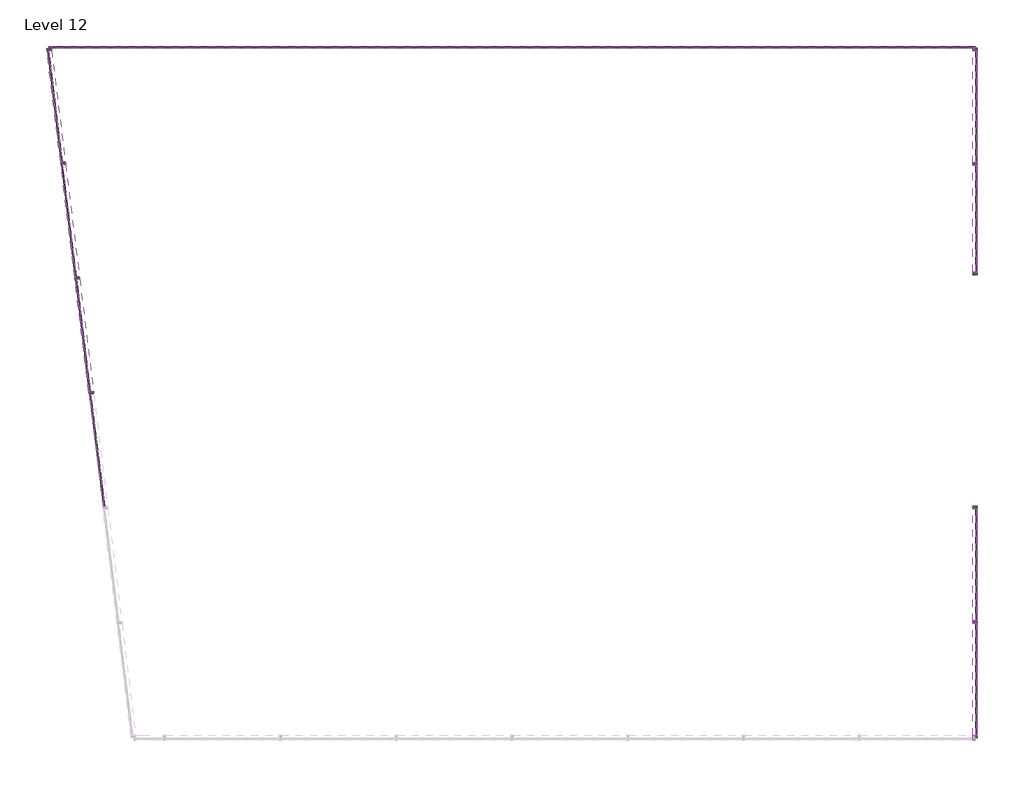
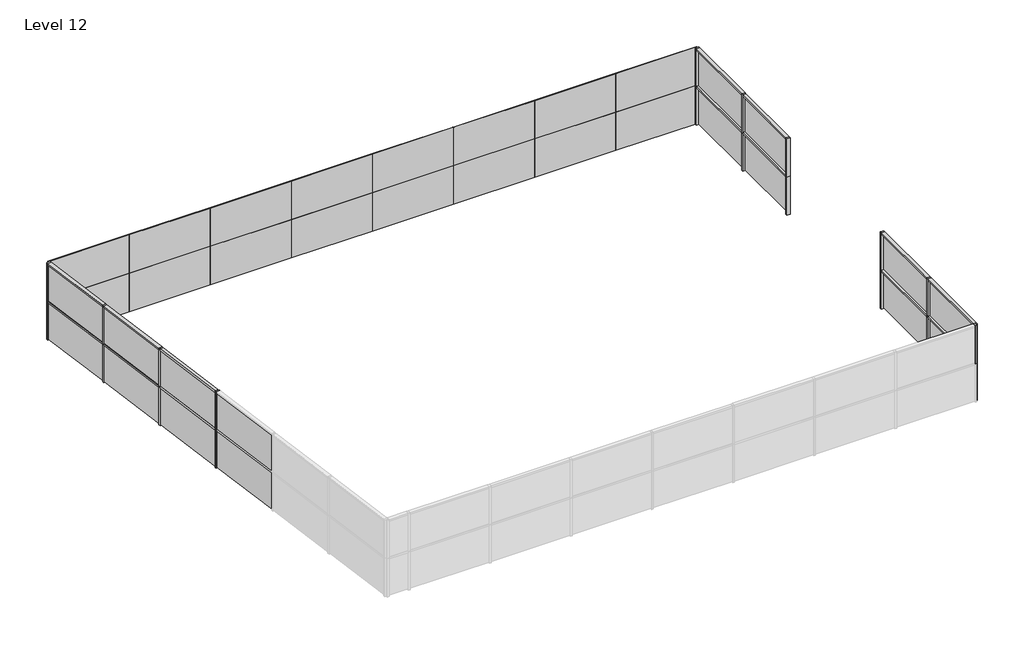
# One storey, part 2 of 2: 35 members, 32 plates.
"""IFC4 building model written with IfcOpenShell, lengths in millimetres."""

from ifc_helpers import new_model, si_unit, origin, place, context, project, spatial, transform, mapped, element, save
from components import member_daa7a266, member_82905deb, member_19d0a4ec, member_8cef0660, member_db480205, member_4491d118, member_46bdb8c2, member_1b94d493, system_panel_glazed_1e57f9bb, system_panel_glazed_37f15d2e, system_panel_glazed_3620f98e, system_panel_glazed_e46d4b42, system_panel_glazed_2a6c68b7, system_panel_glazed_7fb1fc2b, system_panel_glazed_d483336f

model = new_model("IFC4")

# Units and contexts
model_context = context("Model", 3, world=origin())
ifc_project = project(units=[si_unit("LENGTHUNIT", "METRE", prefix="MILLI")], contexts=[model_context])

# Site, building, storey
site = spatial("IfcSite", under=ifc_project)
building = spatial("IfcBuilding", under=site)
storey = spatial("IfcBuildingStorey", under=building, Name="Level 12", Elevation=33528.0)

# Members
placement = place(None, origin())
member_shape = member_daa7a266(model_context)
element("IfcMember", 1, ObjectType="Rectangular Mullion : 2.5\" x 5\" rectangular", at=placement, inside=storey, context=model_context, shape_type="MappedRepresentation", body=[
    mapped(member_shape, transform((-10113.8959567, 8178.7803212, 36576.0), x_axis=(0.0, 0.0, 1.0), y_axis=(-0.9925461516413222, -0.12186934340514613, 0.0), z_axis=(0.12186934340514613, -0.9925461516413222, 0.0))),
])
element("IfcMember", 2, ObjectType="Rectangular Mullion : 2.5\" x 5\" rectangular", at=placement, inside=storey, context=model_context, shape_type="MappedRepresentation", body=[
    mapped(member_shape, transform((13902.5156363, -946.6363705, 36576.0), x_axis=(0.0, 0.0, 1.0), y_axis=(1.0, 0.0, 0.0), z_axis=(0.0, 1.0, 0.0))),
])
element("IfcMember", 3, ObjectType="Rectangular Mullion : 2.5\" x 5\" rectangular", at=placement, inside=storey, context=model_context, shape_type="MappedRepresentation", body=[
    mapped(member_shape, transform((13902.5156363, -3962.8863708, 36576.0), x_axis=(0.0, 0.0, 1.0), y_axis=(1.0, 0.0, 0.0), z_axis=(0.0, 1.0, 0.0))),
])
element("IfcMember", 4, ObjectType="Rectangular Mullion : 2.5\" x 5\" rectangular", at=placement, inside=storey, context=model_context, shape_type="MappedRepresentation", body=[
    mapped(member_shape, transform((13902.5156363, 11109.0476508, 36576.0), x_axis=(0.0, 0.0, 1.0), y_axis=(1.0, 0.0, 0.0), z_axis=(0.0, 1.0, 0.0))),
])
member_2_shape = member_82905deb(model_context)
element("IfcMember", 5, ObjectType="Rectangular Mullion : 2.5\" x 5\" rectangular", at=placement, inside=storey, context=model_context, shape_type="MappedRepresentation", body=[
    mapped(member_2_shape, transform((-9367.1110876, 2096.7056405, 36576.0), x_axis=(-0.1218693434051459, 0.9925461516413222, 0.0), y_axis=(-0.9925461516413222, -0.1218693434051459, 0.0), z_axis=(0.0, 0.0, 1.0))),
])
element("IfcMember", 6, ObjectType="Rectangular Mullion : 2.5\" x 5\" rectangular", at=placement, inside=storey, context=model_context, shape_type="MappedRepresentation", body=[
    mapped(member_2_shape, transform((-9738.5688463, 5121.9863107, 36576.0), x_axis=(-0.1218693434051459, 0.9925461516413222, 0.0), y_axis=(-0.9925461516413222, -0.1218693434051459, 0.0), z_axis=(0.0, 0.0, 1.0))),
])
element("IfcMember", 7, ObjectType="Rectangular Mullion : 2.5\" x 5\" rectangular", at=placement, inside=storey, context=model_context, shape_type="MappedRepresentation", body=[
    mapped(member_2_shape, transform((-10110.026605, 8147.2669809, 36576.0), x_axis=(-0.1218693434051459, 0.9925461516413222, 0.0), y_axis=(-0.9925461516413222, -0.1218693434051459, 0.0), z_axis=(0.0, 0.0, 1.0))),
])
element("IfcMember", 8, ObjectType="Rectangular Mullion : 2.5\" x 5\" rectangular", at=placement, inside=storey, context=model_context, shape_type="MappedRepresentation", body=[
    mapped(member_2_shape, transform((13902.5156363, -3931.1363708, 36576.0), x_axis=(0.0, -1.0, 0.0), y_axis=(1.0, 0.0, 0.0), z_axis=(0.0, 0.0, 1.0))),
])
element("IfcMember", 9, ObjectType="Rectangular Mullion : 2.5\" x 5\" rectangular", at=placement, inside=storey, context=model_context, shape_type="MappedRepresentation", body=[
    mapped(member_2_shape, transform((13902.5156363, 8124.5476505, 36576.0), x_axis=(0.0, -1.0, 0.0), y_axis=(1.0, 0.0, 0.0), z_axis=(0.0, 0.0, 1.0))),
])
member_3_shape = member_19d0a4ec(model_context)
element("IfcMember", 10, ObjectType="Rectangular Mullion : 2.5\" x 5\" rectangular", at=placement, inside=storey, context=model_context, shape_type="MappedRepresentation", body=[
    mapped(member_3_shape, transform((-10113.8959567, 8178.7803212, 35052.0), x_axis=(0.0, 0.0, 1.0), y_axis=(-0.9925461516413222, -0.12186934340514599, 0.0), z_axis=(0.12186934340514599, -0.9925461516413222, 0.0))),
])
element("IfcMember", 11, ObjectType="Rectangular Mullion : 2.5\" x 5\" rectangular", at=placement, inside=storey, context=model_context, shape_type="MappedRepresentation", body=[
    mapped(member_3_shape, transform((13902.5156363, -946.6363705, 35052.0), x_axis=(0.0, 0.0, 1.0), y_axis=(1.0, 0.0, 0.0), z_axis=(0.0, 1.0, 0.0))),
])
element("IfcMember", 12, ObjectType="Rectangular Mullion : 2.5\" x 5\" rectangular", at=placement, inside=storey, context=model_context, shape_type="MappedRepresentation", body=[
    mapped(member_3_shape, transform((13902.5156363, -3962.8863708, 35052.0), x_axis=(0.0, 0.0, 1.0), y_axis=(1.0, 0.0, 0.0), z_axis=(0.0, 1.0, 0.0))),
])
element("IfcMember", 13, ObjectType="Rectangular Mullion : 2.5\" x 5\" rectangular", at=placement, inside=storey, context=model_context, shape_type="MappedRepresentation", body=[
    mapped(member_3_shape, transform((13902.5156363, 11109.0476508, 35052.0), x_axis=(0.0, 0.0, 1.0), y_axis=(1.0, 0.0, 0.0), z_axis=(0.0, 1.0, 0.0))),
])
member_4_shape = member_8cef0660(model_context)
element("IfcMember", 14, ObjectType="Rectangular Mullion : 2.5\" x 5\" rectangular", at=placement, inside=storey, context=model_context, shape_type="MappedRepresentation", body=[
    mapped(member_4_shape, transform((-9370.9804393, 2128.2189808, 35052.0), x_axis=(0.0, 0.0, 1.0), y_axis=(-0.9925461516413222, -0.12186934340514602, 0.0), z_axis=(0.12186934340514602, -0.9925461516413222, 0.0))),
])
element("IfcMember", 15, ObjectType="Rectangular Mullion : 2.5\" x 5\" rectangular", at=placement, inside=storey, context=model_context, shape_type="MappedRepresentation", body=[
    mapped(member_4_shape, transform((-9742.438198, 5153.499651, 35052.0), x_axis=(0.0, 0.0, 1.0), y_axis=(-0.9925461516413222, -0.12186934340514602, 0.0), z_axis=(0.12186934340514602, -0.9925461516413222, 0.0))),
])
member_5_shape = member_db480205(model_context)
element("IfcMember", 16, ObjectType="Rectangular Mullion : 2.5\" x 5\" rectangular", at=placement, inside=storey, context=model_context, shape_type="MappedRepresentation", body=[
    mapped(member_5_shape, transform((-9370.9804393, 2128.2189808, 36576.0), x_axis=(0.0, 0.0, 1.0), y_axis=(-0.9925461516413223, -0.12186934340514563, 0.0), z_axis=(0.12186934340514562, -0.9925461516413222, 0.0))),
])
element("IfcMember", 17, ObjectType="Rectangular Mullion : 2.5\" x 5\" rectangular", at=placement, inside=storey, context=model_context, shape_type="MappedRepresentation", body=[
    mapped(member_5_shape, transform((-9742.438198, 5153.499651, 36576.0), x_axis=(0.0, 0.0, 1.0), y_axis=(-0.9925461516413222, -0.1218693434051461, 0.0), z_axis=(0.1218693434051461, -0.9925461516413222, 0.0))),
])
element("IfcMember", 18, ObjectType="Rectangular Mullion : 2.5\" x 5\" rectangular", at=placement, inside=storey, context=model_context, shape_type="MappedRepresentation", body=[
    mapped(member_2_shape, transform((-9367.1110876, 2096.7056405, 35052.0), x_axis=(-0.1218693434051459, 0.9925461516413222, 0.0), y_axis=(-0.9925461516413222, -0.1218693434051459, 0.0), z_axis=(0.0, 0.0, 1.0))),
])
element("IfcMember", 19, ObjectType="Rectangular Mullion : 2.5\" x 5\" rectangular", at=placement, inside=storey, context=model_context, shape_type="MappedRepresentation", body=[
    mapped(member_2_shape, transform((-9738.5688463, 5121.9863107, 35052.0), x_axis=(-0.1218693434051459, 0.9925461516413222, 0.0), y_axis=(-0.9925461516413222, -0.1218693434051459, 0.0), z_axis=(0.0, 0.0, 1.0))),
])
element("IfcMember", 20, ObjectType="Rectangular Mullion : 2.5\" x 5\" rectangular", at=placement, inside=storey, context=model_context, shape_type="MappedRepresentation", body=[
    mapped(member_2_shape, transform((-10110.026605, 8147.2669809, 35052.0), x_axis=(-0.1218693434051459, 0.9925461516413222, 0.0), y_axis=(-0.9925461516413222, -0.1218693434051459, 0.0), z_axis=(0.0, 0.0, 1.0))),
])
element("IfcMember", 21, ObjectType="Rectangular Mullion : 2.5\" x 5\" rectangular", at=placement, inside=storey, context=model_context, shape_type="MappedRepresentation", body=[
    mapped(member_2_shape, transform((13902.5156363, -3931.1363708, 35052.0), x_axis=(0.0, -1.0, 0.0), y_axis=(1.0, 0.0, 0.0), z_axis=(0.0, 0.0, 1.0))),
])
element("IfcMember", 22, ObjectType="Rectangular Mullion : 2.5\" x 5\" rectangular", at=placement, inside=storey, context=model_context, shape_type="MappedRepresentation", body=[
    mapped(member_2_shape, transform((13902.5156363, 8124.5476505, 35052.0), x_axis=(0.0, -1.0, 0.0), y_axis=(1.0, 0.0, 0.0), z_axis=(0.0, 0.0, 1.0))),
])
member_6_shape = member_4491d118(model_context)
element("IfcMember", 23, ObjectType="Rectangular Mullion : 2.5\" x 5\" rectangular", at=placement, inside=storey, context=model_context, shape_type="MappedRepresentation", body=[
    mapped(member_6_shape, transform((-10481.4843637, 11172.5476508, 36576.0), x_axis=(-0.1218693434051459, 0.9925461516413222, 0.0), y_axis=(-0.9925461516413222, -0.1218693434051459, 0.0), z_axis=(0.0, 0.0, 1.0))),
])
element("IfcMember", 24, ObjectType="Rectangular Mullion : 2.5\" x 5\" rectangular", at=placement, inside=storey, context=model_context, shape_type="MappedRepresentation", body=[
    mapped(member_6_shape, transform((13902.5156363, -6979.1363705, 36576.0), x_axis=(0.0, -1.0, 0.0), y_axis=(1.0, 0.0, 0.0), z_axis=(0.0, 0.0, 1.0))),
])
element("IfcMember", 25, ObjectType="Rectangular Mullion : 2.5\" x 5\" rectangular", at=placement, inside=storey, context=model_context, shape_type="MappedRepresentation", body=[
    mapped(member_6_shape, transform((13902.5156363, 5212.8636295, 36576.0), x_axis=(0.0, -1.0, 0.0), y_axis=(1.0, 0.0, 0.0), z_axis=(0.0, 0.0, 1.0))),
])
element("IfcMember", 26, ObjectType="Rectangular Mullion : 2.5\" x 5\" rectangular", at=placement, inside=storey, context=model_context, shape_type="MappedRepresentation", body=[
    mapped(member_6_shape, transform((13902.5156363, -883.1363705, 33528.0), x_axis=(0.0, 1.0, 0.0), y_axis=(1.0, 0.0, 0.0), z_axis=(0.0, 0.0, -1.0))),
])
element("IfcMember", 27, ObjectType="Rectangular Mullion : 2.5\" x 5\" rectangular", at=placement, inside=storey, context=model_context, shape_type="MappedRepresentation", body=[
    mapped(member_6_shape, transform((13902.5156363, 11172.5476508, 33528.0), x_axis=(0.0, 1.0, 0.0), y_axis=(1.0, 0.0, 0.0), z_axis=(0.0, 0.0, -1.0))),
])
element("IfcMember", 28, ObjectType="Rectangular Mullion : 2.5\" x 5\" rectangular", at=placement, inside=storey, context=model_context, shape_type="MappedRepresentation", body=[
    mapped(member_6_shape, transform((13902.5156363, -6979.1363705, 35052.0), x_axis=(1.0, 0.0, 0.0), y_axis=(0.0, -1.0, 0.0), z_axis=(0.0, 0.0, -1.0))),
])
element("IfcMember", 29, ObjectType="Rectangular Mullion : 2.5\" x 5\" rectangular", at=placement, inside=storey, context=model_context, shape_type="MappedRepresentation", body=[
    mapped(member_6_shape, transform((13902.5156363, -883.1363705, 35052.0), x_axis=(0.0, 1.0, 0.0), y_axis=(1.0, 0.0, 0.0), z_axis=(0.0, 0.0, -1.0))),
])
element("IfcMember", 30, ObjectType="Rectangular Mullion : 2.5\" x 5\" rectangular", at=placement, inside=storey, context=model_context, shape_type="MappedRepresentation", body=[
    mapped(member_6_shape, transform((13902.5156363, 11172.5476508, 35052.0), x_axis=(0.0, 1.0, 0.0), y_axis=(1.0, 0.0, 0.0), z_axis=(0.0, 0.0, -1.0))),
])
element("IfcMember", 31, ObjectType="Rectangular Mullion : 2.5\" x 5\" rectangular", at=placement, inside=storey, context=model_context, shape_type="MappedRepresentation", body=[
    mapped(member_6_shape, transform((-10481.4843637, 11172.5476508, 35052.0), x_axis=(-0.1218693434051459, 0.9925461516413222, 0.0), y_axis=(-0.9925461516413222, -0.1218693434051459, 0.0), z_axis=(0.0, 0.0, 1.0))),
])
element("IfcMember", 32, ObjectType="Rectangular Mullion : 2.5\" x 5\" rectangular", at=placement, inside=storey, context=model_context, shape_type="MappedRepresentation", body=[
    mapped(member_6_shape, transform((13902.5156363, -6979.1363705, 35052.0), x_axis=(0.0, -1.0, 0.0), y_axis=(1.0, 0.0, 0.0), z_axis=(0.0, 0.0, 1.0))),
])
element("IfcMember", 33, ObjectType="Rectangular Mullion : 2.5\" x 5\" rectangular", at=placement, inside=storey, context=model_context, shape_type="MappedRepresentation", body=[
    mapped(member_6_shape, transform((13902.5156363, 5212.8636295, 35052.0), x_axis=(0.0, -1.0, 0.0), y_axis=(1.0, 0.0, 0.0), z_axis=(0.0, 0.0, 1.0))),
])
member_7_shape = member_46bdb8c2(model_context)
element("IfcMember", 34, ObjectType="Rectangular Mullion : 2.5\" x 5\" rectangular", at=placement, inside=storey, context=model_context, shape_type="MappedRepresentation", body=[
    mapped(member_7_shape, transform((13902.5156363, 8092.7976505, 35052.0), x_axis=(0.0, 0.0, 1.0), y_axis=(1.0, 0.0, 0.0), z_axis=(0.0, 1.0, 0.0))),
])
member_8_shape = member_1b94d493(model_context)
element("IfcMember", 35, ObjectType="Rectangular Mullion : 2.5\" x 5\" rectangular", at=placement, inside=storey, context=model_context, shape_type="MappedRepresentation", body=[
    mapped(member_8_shape, transform((13902.5156363, 8092.7976505, 36576.0), x_axis=(0.0, 0.0, 1.0), y_axis=(1.0, 0.0, 0.0), z_axis=(0.0, 1.0, 0.0))),
])

# Plates
system_panel_glazed_shape = system_panel_glazed_1e57f9bb(model_context)
element("IfcPlate", 36, ObjectType="System Panel : Glazed", at=placement, inside=storey, context=model_context, shape_type="MappedRepresentation", body=[
    mapped(system_panel_glazed_shape, transform((-8957.4843636, 11172.5476508, 33528.0), x_axis=(1.0, 0.0, 0.0), y_axis=(0.0, 1.0, 0.0), z_axis=(0.0, 0.0, 1.0))),
])
element("IfcPlate", 37, ObjectType="System Panel : Glazed", at=placement, inside=storey, context=model_context, shape_type="MappedRepresentation", body=[
    mapped(system_panel_glazed_shape, transform((-5909.4843634, 11172.5476508, 33528.0), x_axis=(1.0, 0.0, 0.0), y_axis=(0.0, 1.0, 0.0), z_axis=(0.0, 0.0, 1.0))),
])
element("IfcPlate", 38, ObjectType="System Panel : Glazed", at=placement, inside=storey, context=model_context, shape_type="MappedRepresentation", body=[
    mapped(system_panel_glazed_shape, transform((-2861.4843634, 11172.5476508, 33528.0), x_axis=(1.0, 0.0, 0.0), y_axis=(0.0, 1.0, 0.0), z_axis=(0.0, 0.0, 1.0))),
])
element("IfcPlate", 39, ObjectType="System Panel : Glazed", at=placement, inside=storey, context=model_context, shape_type="MappedRepresentation", body=[
    mapped(system_panel_glazed_shape, transform((186.5156366, 11172.5476508, 33528.0), x_axis=(1.0, 0.0, 0.0), y_axis=(0.0, 1.0, 0.0), z_axis=(0.0, 0.0, 1.0))),
])
element("IfcPlate", 40, ObjectType="System Panel : Glazed", at=placement, inside=storey, context=model_context, shape_type="MappedRepresentation", body=[
    mapped(system_panel_glazed_shape, transform((3234.5156366, 11172.5476508, 33528.0), x_axis=(1.0, 0.0, 0.0), y_axis=(0.0, 1.0, 0.0), z_axis=(0.0, 0.0, 1.0))),
])
element("IfcPlate", 41, ObjectType="System Panel : Glazed", at=placement, inside=storey, context=model_context, shape_type="MappedRepresentation", body=[
    mapped(system_panel_glazed_shape, transform((6282.5156366, 11172.5476508, 33528.0), x_axis=(1.0, 0.0, 0.0), y_axis=(0.0, 1.0, 0.0), z_axis=(0.0, 0.0, 1.0))),
])
element("IfcPlate", 42, ObjectType="System Panel : Glazed", at=placement, inside=storey, context=model_context, shape_type="MappedRepresentation", body=[
    mapped(system_panel_glazed_shape, transform((9330.5156366, 11172.5476508, 33528.0), x_axis=(1.0, 0.0, 0.0), y_axis=(0.0, 1.0, 0.0), z_axis=(0.0, 0.0, 1.0))),
])
element("IfcPlate", 43, ObjectType="System Panel : Glazed", at=placement, inside=storey, context=model_context, shape_type="MappedRepresentation", body=[
    mapped(system_panel_glazed_shape, transform((12378.5156364, 11172.5476508, 33528.0), x_axis=(1.0, 0.0, 0.0), y_axis=(0.0, 1.0, 0.0), z_axis=(0.0, 0.0, 1.0))),
])
element("IfcPlate", 44, ObjectType="System Panel : Glazed", at=placement, inside=storey, context=model_context, shape_type="MappedRepresentation", body=[
    mapped(system_panel_glazed_shape, transform((-8957.4843636, 11172.5476508, 35052.0), x_axis=(1.0, 0.0, 0.0), y_axis=(0.0, 1.0, 0.0), z_axis=(0.0, 0.0, 1.0))),
])
element("IfcPlate", 45, ObjectType="System Panel : Glazed", at=placement, inside=storey, context=model_context, shape_type="MappedRepresentation", body=[
    mapped(system_panel_glazed_shape, transform((-5909.4843634, 11172.5476508, 35052.0), x_axis=(1.0, 0.0, 0.0), y_axis=(0.0, 1.0, 0.0), z_axis=(0.0, 0.0, 1.0))),
])
element("IfcPlate", 46, ObjectType="System Panel : Glazed", at=placement, inside=storey, context=model_context, shape_type="MappedRepresentation", body=[
    mapped(system_panel_glazed_shape, transform((-2861.4843634, 11172.5476508, 35052.0), x_axis=(1.0, 0.0, 0.0), y_axis=(0.0, 1.0, 0.0), z_axis=(0.0, 0.0, 1.0))),
])
element("IfcPlate", 47, ObjectType="System Panel : Glazed", at=placement, inside=storey, context=model_context, shape_type="MappedRepresentation", body=[
    mapped(system_panel_glazed_shape, transform((186.5156366, 11172.5476508, 35052.0), x_axis=(1.0, 0.0, 0.0), y_axis=(0.0, 1.0, 0.0), z_axis=(0.0, 0.0, 1.0))),
])
element("IfcPlate", 48, ObjectType="System Panel : Glazed", at=placement, inside=storey, context=model_context, shape_type="MappedRepresentation", body=[
    mapped(system_panel_glazed_shape, transform((3234.5156366, 11172.5476508, 35052.0), x_axis=(1.0, 0.0, 0.0), y_axis=(0.0, 1.0, 0.0), z_axis=(0.0, 0.0, 1.0))),
])
element("IfcPlate", 49, ObjectType="System Panel : Glazed", at=placement, inside=storey, context=model_context, shape_type="MappedRepresentation", body=[
    mapped(system_panel_glazed_shape, transform((6282.5156366, 11172.5476508, 35052.0), x_axis=(1.0, 0.0, 0.0), y_axis=(0.0, 1.0, 0.0), z_axis=(0.0, 0.0, 1.0))),
])
element("IfcPlate", 50, ObjectType="System Panel : Glazed", at=placement, inside=storey, context=model_context, shape_type="MappedRepresentation", body=[
    mapped(system_panel_glazed_shape, transform((9330.5156366, 11172.5476508, 35052.0), x_axis=(1.0, 0.0, 0.0), y_axis=(0.0, 1.0, 0.0), z_axis=(0.0, 0.0, 1.0))),
])
element("IfcPlate", 51, ObjectType="System Panel : Glazed", at=placement, inside=storey, context=model_context, shape_type="MappedRepresentation", body=[
    mapped(system_panel_glazed_shape, transform((12378.5156364, 11172.5476508, 35052.0), x_axis=(1.0, 0.0, 0.0), y_axis=(0.0, 1.0, 0.0), z_axis=(0.0, 0.0, 1.0))),
])
system_panel_glazed_2_shape = system_panel_glazed_37f15d2e(model_context)
element("IfcPlate", 52, ObjectType="System Panel : Glazed", at=placement, inside=storey, context=model_context, shape_type="MappedRepresentation", body=[
    mapped(system_panel_glazed_2_shape, transform((-10293.8208085, 9644.1506457, 35083.75), x_axis=(-0.1218693434051459, 0.9925461516413222, 0.0), y_axis=(-0.9925461516413222, -0.1218693434051459, 0.0), z_axis=(0.0, 0.0, 1.0))),
])
element("IfcPlate", 53, ObjectType="System Panel : Glazed", at=placement, inside=storey, context=model_context, shape_type="MappedRepresentation", body=[
    mapped(system_panel_glazed_2_shape, transform((13902.5156363, -2423.0113706, 35083.75), x_axis=(0.0, -1.0, 0.0), y_axis=(1.0, 0.0, 0.0), z_axis=(0.0, 0.0, 1.0))),
])
element("IfcPlate", 54, ObjectType="System Panel : Glazed", at=placement, inside=storey, context=model_context, shape_type="MappedRepresentation", body=[
    mapped(system_panel_glazed_2_shape, transform((13902.5156363, -5439.2613706, 35083.75), x_axis=(0.0, -1.0, 0.0), y_axis=(1.0, 0.0, 0.0), z_axis=(0.0, 0.0, 1.0))),
])
element("IfcPlate", 55, ObjectType="System Panel : Glazed", at=placement, inside=storey, context=model_context, shape_type="MappedRepresentation", body=[
    mapped(system_panel_glazed_2_shape, transform((13902.5156363, 9632.6726506, 35083.75), x_axis=(0.0, -1.0, 0.0), y_axis=(1.0, 0.0, 0.0), z_axis=(0.0, 0.0, 1.0))),
])
system_panel_glazed_3_shape = system_panel_glazed_3620f98e(model_context)
element("IfcPlate", 56, ObjectType="System Panel : Glazed", at=placement, inside=storey, context=model_context, shape_type="MappedRepresentation", body=[
    mapped(system_panel_glazed_3_shape, transform((-9181.3822083, 584.0653054, 35083.75), x_axis=(-0.1218693434051459, 0.9925461516413222, 0.0), y_axis=(-0.9925461516413222, -0.1218693434051459, 0.0), z_axis=(0.0, 0.0, 1.0))),
])
element("IfcPlate", 57, ObjectType="System Panel : Glazed", at=placement, inside=storey, context=model_context, shape_type="MappedRepresentation", body=[
    mapped(system_panel_glazed_3_shape, transform((-9552.839967, 3609.3459756, 35083.75), x_axis=(-0.1218693434051459, 0.9925461516413222, 0.0), y_axis=(-0.9925461516413222, -0.1218693434051459, 0.0), z_axis=(0.0, 0.0, 1.0))),
])
element("IfcPlate", 58, ObjectType="System Panel : Glazed", at=placement, inside=storey, context=model_context, shape_type="MappedRepresentation", body=[
    mapped(system_panel_glazed_3_shape, transform((-9924.2977257, 6634.6266458, 35083.75), x_axis=(-0.1218693434051459, 0.9925461516413222, 0.0), y_axis=(-0.9925461516413222, -0.1218693434051459, 0.0), z_axis=(0.0, 0.0, 1.0))),
])
system_panel_glazed_4_shape = system_panel_glazed_e46d4b42(model_context)
element("IfcPlate", 59, ObjectType="System Panel : Glazed", at=placement, inside=storey, context=model_context, shape_type="MappedRepresentation", body=[
    mapped(system_panel_glazed_4_shape, transform((-10293.8208085, 9644.1506457, 33559.75), x_axis=(-0.1218693434051459, 0.9925461516413222, 0.0), y_axis=(-0.9925461516413222, -0.1218693434051459, 0.0), z_axis=(0.0, 0.0, 1.0))),
])
element("IfcPlate", 60, ObjectType="System Panel : Glazed", at=placement, inside=storey, context=model_context, shape_type="MappedRepresentation", body=[
    mapped(system_panel_glazed_4_shape, transform((13902.5156363, -2423.0113706, 33559.75), x_axis=(0.0, -1.0, 0.0), y_axis=(1.0, 0.0, 0.0), z_axis=(0.0, 0.0, 1.0))),
])
element("IfcPlate", 61, ObjectType="System Panel : Glazed", at=placement, inside=storey, context=model_context, shape_type="MappedRepresentation", body=[
    mapped(system_panel_glazed_4_shape, transform((13902.5156363, -5439.2613706, 33559.75), x_axis=(0.0, -1.0, 0.0), y_axis=(1.0, 0.0, 0.0), z_axis=(0.0, 0.0, 1.0))),
])
element("IfcPlate", 62, ObjectType="System Panel : Glazed", at=placement, inside=storey, context=model_context, shape_type="MappedRepresentation", body=[
    mapped(system_panel_glazed_4_shape, transform((13902.5156363, 9632.6726506, 33559.75), x_axis=(0.0, -1.0, 0.0), y_axis=(1.0, 0.0, 0.0), z_axis=(0.0, 0.0, 1.0))),
])
system_panel_glazed_5_shape = system_panel_glazed_2a6c68b7(model_context)
element("IfcPlate", 63, ObjectType="System Panel : Glazed", at=placement, inside=storey, context=model_context, shape_type="MappedRepresentation", body=[
    mapped(system_panel_glazed_5_shape, transform((-9181.3822083, 584.0653054, 33559.75), x_axis=(-0.1218693434051459, 0.9925461516413222, 0.0), y_axis=(-0.9925461516413222, -0.1218693434051459, 0.0), z_axis=(0.0, 0.0, 1.0))),
])
element("IfcPlate", 64, ObjectType="System Panel : Glazed", at=placement, inside=storey, context=model_context, shape_type="MappedRepresentation", body=[
    mapped(system_panel_glazed_5_shape, transform((-9552.839967, 3609.3459756, 33559.75), x_axis=(-0.1218693434051459, 0.9925461516413222, 0.0), y_axis=(-0.9925461516413222, -0.1218693434051459, 0.0), z_axis=(0.0, 0.0, 1.0))),
])
element("IfcPlate", 65, ObjectType="System Panel : Glazed", at=placement, inside=storey, context=model_context, shape_type="MappedRepresentation", body=[
    mapped(system_panel_glazed_5_shape, transform((-9924.2977257, 6634.6266458, 33559.75), x_axis=(-0.1218693434051459, 0.9925461516413222, 0.0), y_axis=(-0.9925461516413222, -0.1218693434051459, 0.0), z_axis=(0.0, 0.0, 1.0))),
])
system_panel_glazed_6_shape = system_panel_glazed_7fb1fc2b(model_context)
element("IfcPlate", 66, ObjectType="System Panel : Glazed", at=placement, inside=storey, context=model_context, shape_type="MappedRepresentation", body=[
    mapped(system_panel_glazed_6_shape, transform((13902.5156363, 6684.58064, 35083.75), x_axis=(0.0, -1.0, 0.0), y_axis=(1.0, 0.0, 0.0), z_axis=(0.0, 0.0, 1.0))),
])
system_panel_glazed_7_shape = system_panel_glazed_d483336f(model_context)
element("IfcPlate", 67, ObjectType="System Panel : Glazed", at=placement, inside=storey, context=model_context, shape_type="MappedRepresentation", body=[
    mapped(system_panel_glazed_7_shape, transform((13902.5156363, 6684.58064, 33559.75), x_axis=(0.0, -1.0, 0.0), y_axis=(1.0, 0.0, 0.0), z_axis=(0.0, 0.0, 1.0))),
])

save(model, "model.ifc")

# Revit data of these elements
# Type "Rectangular Mullion : 2.5\" x 5\" rectangular"
#   built-in parameter 1007304 = 0.416667 (stored number, unit not read)
#   built-in parameter 1007301 = 0.104167 (stored number, unit not read)
#   built-in parameter 1007300 = 0.104167 (stored number, unit not read)
# Type "System Panel : Glazed"
#   Construction Type Id = "GSP4R"
#   Analytic Construction = "1/8 in Pilkington single glazing"
#   Visual Light Transmittance = 0.9
#   Solar Heat Gain Coefficient = 0.86
#   Heat Transfer Coefficient (U) = 1.18115 BTU/(h·ft²·°F)
#   Define Thermal Properties by = 1
# Elements 1, 2, 3, 4, 5, 6, 7, 8, 9, 10, 11, 12, 13, 14, 15, 16, 17, 18, 19, 20, 21, 22, 23, 24, 25, 26, 27, 28, 29, 30, 31, 32, 33, 34, 35 (IfcMember, "Rectangular Mullion : 2.5\" x 5\" rectangular")
#   Phase Created = New Construction
#   Materials on its faces: "Aluminum"
# Elements 36, 37, 38, 39, 40, 41, 42, 43, 44, 45, 46, 47, 48, 49, 50, 51, 52, 53, 54, 55, 56, 57, 58, 59, 60, 61, 62, 63, 64, 65, 66, 67 (IfcPlate, "System Panel : Glazed")
#   Phase Created = New Construction
#   Materials on its faces: "Glass"
# Materials
#   "Aluminum": class "Metal", colour RGB 247 247 247, transparency 0, Description = "Aluminum 6061", Cost = 0
#   "Glass": class "Glass", colour RGB 0 128 192, transparency 0.75, Description = "Soda Lime Glass", Cost = 0
